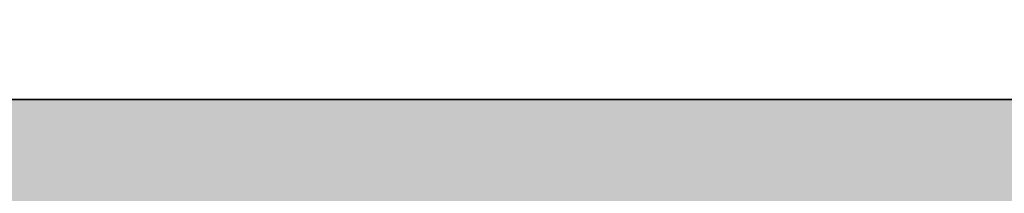
# Model space of a CAD drawing. Units: inches. Extents: x 2091 to 2899, y 967 to 2217.
# Tile 85 of 256: x 2251.283145 to 2251.287593, y 1099.918635 to 1099.919418. Entities that reach past the tile are written whole.
import ezdxf

# ---------------------------------------------------------------- set-up
doc = ezdxf.new("R2010")
doc.units = ezdxf.units.IN
doc.layers.add('A-WALL-PATT', color=141, linetype='Continuous', lineweight=13, true_color=0xadddf7)
doc.layers.add('L-SITE-WALL', color=7, linetype='Continuous', lineweight=35)

msp = doc.modelspace()

# ---------------------------------------------------------------- hatches: boundary and pattern name
at = {"layer": 'A-WALL-PATT'}
h = msp.add_hatch(color=256, dxfattribs=at)
h.dxf.hatch_style = 1
h.paths.add_polyline_path([(2212.1436027, 1941.4190588), (2387.6436027, 1941.4190588), (2387.6436027, 1824.4190588), (2392.1436027, 1824.4190588), (2392.1436027, 1941.4190588), (2609.6436027, 1941.4190588), (2609.6436027, 1825.9190588), (2614.1436027, 1825.9190588), (2614.1436027, 1941.4190588), (2794.1436027, 1941.4190588), (2794.1436027, 1928.7621663), (2803.1436027, 1928.7621663), (2803.1436027, 2050.9190588), (2203.1436027, 2050.9190588), (2203.1436027, 1900.7578592), (2212.1436027, 1900.7578592)])
h.paths.add_polyline_path([(2212.1436027, 1945.9190588), (2212.1436027, 2041.9190588), (2794.1436027, 2041.9190588), (2794.1436027, 1945.9190588), (2402.2482445, 1945.9190588), (2401.1024337, 1945.7758325), (2398.7024337, 1945.7758325)], flags=16)
h.paths.add_polyline_path([(2230.2298609, 1948.0627926), (2227.3498609, 1949.5027926), (2225.9098609, 1951.9027926), (2223.9898609, 1952.8627926), (2223.0298609, 1955.2627926), (2222.0698609, 1959.5827926), (2222.0698609, 1963.4227926), (2223.0298609, 1965.6627926), (2223.9898609, 1965.3427926), (2225.58591, 1963.860747), (2226.9115333, 1964.9572589), (2226.9488609, 1965.9387926), (2227.7783187, 1966.9521426), (2228.1999161, 1968.8787044), (2230.7098609, 1964.8627926), (2233.5898609, 1966.3027926), (2233.607309, 1966.3318728), (2233.7726595, 1964.9382048), (2234.6338015, 1963.6764729), (2235.0298609, 1963.9027926), (2236.2820348, 1965.5723578), (2235.9898609, 1962.9427926), (2237.9545121, 1957.5400019), (2238.3898609, 1957.9027926), (2239.2158609, 1960.3057926), (2238.6545655, 1966.3849599), (2238.6927918, 1966.4380694), (2238.8405779, 1967.4997069), (2238.7802908, 1967.6874864), (2238.8805378, 1967.7867629), (2238.6668609, 1966.2517926), (2239.2158609, 1960.3057926), (2238.3898609, 1957.9027926), (2236.9498609, 1956.7027926), (2234.5498609, 1949.9827926)], flags=0)
h.paths.add_polyline_path([(2278.0119735, 1948.0627926), (2276.4964266, 1947.8733492), (2275.8498328, 1947.6886081), (2274.6519735, 1947.1027926)], flags=0)
h.paths.add_polyline_path([(2269.8519735, 1955.7427926), (2268.2761762, 1956.6293287), (2270.8673022, 1956.3483982), (2269.3719735, 1958.1427926), (2268.7149641, 1959.1923253), (2270.5698328, 1958.7286081), (2268.5807252, 1961.9060872), (2270.8119735, 1960.8918835), (2270.8119735, 1963.4227926), (2271.3933148, 1964.7792556), (2270.2917623, 1966.1561963), (2271.7719735, 1965.6627926), (2272.1413868, 1966.5247568), (2273.9298328, 1965.9286081), (2275.6303855, 1968.054299), (2276.331938, 1966.72186), (2276.5204313, 1966.9521426), (2276.9420286, 1968.8787044), (2277.7342926, 1967.6110821), (2278.1398879, 1969.4645199), (2279.6591239, 1967.0337425), (2280.4119735, 1966.7827926), (2280.9493019, 1967.5887851), (2281.6098328, 1967.3686081), (2282.1332658, 1968.1537576), (2282.3492351, 1966.3334449), (2282.3498491, 1966.3325853), (2283.40755, 1968.0954201), (2283.7126314, 1965.5240203), (2284.3202211, 1964.6337894), (2284.5118085, 1964.8892393), (2284.2349735, 1965.7047926), (2284.500472, 1967.3189584), (2284.9079444, 1965.4174205), (2285.3963134, 1966.0685791), (2285.4328328, 1966.2906081), (2285.4733384, 1966.1712791), (2286.3539194, 1967.345387), (2286.2220067, 1966.1581734), (2287.6634921, 1968.0801538), (2287.7139735, 1968.4427926), (2288.4815994, 1969.0166793), (2288.5739928, 1968.7288966), (2288.9174612, 1969.0690403), (2288.6068328, 1966.8376081), (2288.9287261, 1963.3513103), (2288.9349735, 1963.3567926), (2288.9297314, 1963.3404224), (2289.015281, 1962.4138692), (2290.1112234, 1963.8751258), (2290.1328328, 1963.9426081), (2290.2176723, 1964.0170576), (2290.1112234, 1963.8751258), (2289.1558328, 1960.8916081), (2288.5940356, 1959.2572271), (2288.5719735, 1959.1027926), (2289.5319735, 1960.5427926), (2290.0119735, 1962.4627926), (2290.1918401, 1962.6426592), (2289.7698328, 1959.6886081), (2286.8898328, 1957.2886081), (2284.4898328, 1950.5686081), (2283.3146576, 1950.046308), (2283.2919735, 1949.9827926), (2280.2900585, 1948.6486081), (2281.1298328, 1948.6486081), (2282.5698328, 1948.1686081), (2283.2047262, 1948.0627926), (2278.9719735, 1948.0627926), (2276.0919735, 1949.5027926), (2274.6519735, 1951.9027926), (2272.7319735, 1952.8627926)], flags=0)
h.paths.add_polyline_path([(2271.1588684, 1958.0217654), (2272.9698328, 1955.8486081), (2272.0098328, 1960.1686081), (2272.0098328, 1964.0086081), (2272.6244258, 1965.4426583), (2274.3280226, 1963.860747), (2275.6536458, 1964.9572589), (2275.6377429, 1964.5390903), (2277.4122311, 1966.0068885), (2277.0329735, 1965.1567926), (2276.829924, 1964.9755966), (2276.7660116, 1963.2950136), (2277.4496351, 1962.6602203), (2279.4519735, 1964.8627926), (2282.3319735, 1966.3027926), (2283.5298328, 1966.8886081), (2283.2945117, 1966.7709476), (2283.9129934, 1963.8846999), (2284.8992493, 1964.4482747), (2284.7319735, 1962.9427926), (2286.6966247, 1957.5400019), (2287.1319735, 1957.9027926), (2287.5419128, 1959.0953883), (2287.7793955, 1958.4423109), (2285.6827383, 1956.6950966), (2285.8765033, 1959.7953357), (2284.7319735, 1962.9427926), (2284.8992493, 1964.4482747), (2283.9129934, 1963.8846999), (2284.2238328, 1962.4341157), (2283.4243649, 1963.6054836), (2281.6098328, 1962.5686081), (2281.1298328, 1960.1686081), (2282.0898328, 1956.3286081), (2283.0498328, 1952.9686081), (2282.5698328, 1950.5686081), (2280.1698328, 1948.6486081), (2279.883316, 1948.7918666), (2278.9719735, 1948.0627926), (2278.9719735, 1949.0227926), (2278.6723132, 1949.3973679), (2277.2898328, 1950.0886081), (2275.8498328, 1952.4886081), (2273.9298328, 1953.4486081), (2272.4898328, 1954.8886081), (2271.9216473, 1954.8886081), (2271.7719735, 1955.2627926)], flags=0)
h.paths.add_polyline_path([(2311.994146, 1955.7427926), (2312.0627174, 1955.6742211), (2312.0550999, 1955.7085002)], flags=0)
h.paths.add_polyline_path([(2331.956146, 1963.9517926), (2333.396146, 1965.3917926), (2331.077146, 1963.3567926), (2330.998603, 1963.1115166)], flags=0)
h.paths.add_polyline_path([(2310.554146, 1954.3027926), (2307.0398066, 1956.2799434), (2310.7629029, 1955.8762843), (2312.474146, 1953.8227926), (2313.434146, 1951.4227926), (2315.354146, 1950.4627926), (2316.794146, 1948.0627926), (2317.466146, 1947.7267926), (2319.3686915, 1947.9646108), (2317.754146, 1949.9827926), (2317.5695306, 1950.6104849), (2316.794146, 1951.9027926), (2314.874146, 1952.8627926), (2313.914146, 1955.2627926), (2311.514146, 1958.1427926), (2309.3754889, 1961.5591681), (2311.514146, 1960.3370783), (2311.514146, 1961.9827926), (2310.6046723, 1963.1196347), (2311.726605, 1962.4785303), (2312.4183321, 1964.09256), (2312.2559642, 1964.2955198), (2313.194146, 1963.9827926), (2313.914146, 1965.6627926), (2314.6467776, 1965.418582), (2315.354146, 1966.3027926), (2316.794146, 1967.7427926), (2316.1574354, 1966.9469043), (2317.0341105, 1965.28186), (2317.2226038, 1965.5121426), (2317.7770481, 1968.0457711), (2318.4741105, 1966.72186), (2318.6626038, 1966.9521426), (2319.0842012, 1968.8787044), (2321.2070492, 1965.4821474), (2322.1614187, 1966.9137017), (2322.554146, 1966.7827926), (2322.7859877, 1967.1305552), (2322.881646, 1966.3242926), (2323.3120408, 1965.7217399), (2323.6512889, 1965.891364), (2324.3964998, 1967.1333822), (2324.6569446, 1964.9382048), (2324.971986, 1964.476611), (2325.3872804, 1967.001499), (2325.9408127, 1964.4183481), (2327.2289286, 1966.1358361), (2327.1663199, 1965.5723578), (2328.0591386, 1966.7627827), (2328.2245759, 1966.2474864), (2329.6679714, 1967.6769101), (2329.6645759, 1967.6874864), (2329.7648229, 1967.7867629), (2329.551146, 1966.2517926), (2330.100146, 1960.3057926), (2329.3328143, 1958.0734703), (2329.3130649, 1957.935225), (2329.634146, 1958.2027926), (2330.234146, 1959.1027926), (2330.714146, 1961.0227926), (2331.034146, 1961.3427926), (2330.714146, 1959.1027926), (2329.634146, 1958.2027926), (2329.274146, 1957.6627926), (2327.7121121, 1956.3610977), (2325.434146, 1949.9827926), (2324.3337687, 1949.493736), (2323.994146, 1948.5427926), (2319.674146, 1946.6227926), (2316.794146, 1948.0627926), (2315.354146, 1950.4627926), (2313.434146, 1951.4227926)], flags=0)
h.paths.add_polyline_path([(2321.3356845, 1947.9520233), (2321.114146, 1948.0627926), (2321.114146, 1949.0227926), (2319.194146, 1951.4227926), (2316.794146, 1959.5827926), (2316.6632369, 1959.5827926), (2315.354146, 1958.1427926), (2314.394146, 1958.1427926), (2313.1483033, 1958.7090847), (2312.954146, 1959.5827926), (2312.954146, 1960.8918835), (2315.834146, 1959.5827926), (2316.6632369, 1959.5827926), (2317.3147094, 1960.2994123), (2315.0301951, 1962.420747), (2316.3558184, 1963.5172589), (2316.3723369, 1963.9516153), (2316.4701951, 1963.860747), (2317.7958184, 1964.9572589), (2317.7552187, 1963.8896871), (2319.175146, 1965.1567926), (2319.4984065, 1965.8813724), (2321.114146, 1965.3427926), (2323.2358851, 1962.3723578), (2325.6863494, 1963.7726231), (2325.5427886, 1962.4805756), (2325.1987827, 1963.4940135), (2324.4785097, 1963.0824289), (2324.9260053, 1960.9941157), (2324.0780866, 1962.2364729), (2322.4147912, 1961.2860184), (2322.074146, 1959.5827926), (2323.034146, 1955.7427926), (2323.994146, 1952.3827926), (2323.514146, 1949.9827926), (2322.1427174, 1948.8856497), (2322.074146, 1948.5427926)], flags=0)
h.paths.add_polyline_path([(2320.2074794, 1963.3374592), (2320.154146, 1963.4227926), (2320.394146, 1963.5427926)], flags=0)
h.paths.add_polyline_path([(2353.8505274, 1965.8105004), (2354.0305274, 1965.7505004), (2354.3305274, 1966.4505004), (2354.3305274, 1966.9305004)], flags=0)
h.paths.add_polyline_path([(2359.0205825, 1969.0264122), (2359.0983824, 1968.9019323), (2359.2335274, 1969.5195004), (2359.2335274, 1969.9995004)], flags=0)
h.paths.add_polyline_path([(2358.2566937, 1966.6816724), (2357.983601, 1966.3480346), (2358.211267, 1966.1461745), (2358.4104918, 1966.3895678)], flags=0)
h.paths.add_polyline_path([(2357.7684731, 1966.0587777), (2357.7321997, 1965.1049667), (2357.751047, 1965.1205565), (2357.7695274, 1965.6065004), (2357.7695274, 1966.057843)], flags=0)
h.paths.add_polyline_path([(2359.1115274, 1965.3045004), (2359.1115274, 1964.8245004), (2359.8445274, 1966.4675004), (2359.8445274, 1966.9475004)], flags=0)
h.paths.add_polyline_path([(2360.2236843, 1966.6214493), (2360.6985274, 1969.3625004), (2360.6985274, 1969.8425004), (2360.2105274, 1967.0255004), (2360.2105274, 1966.6425004)], flags=0)
h.paths.add_polyline_path([(2363.4505274, 1967.8905004), (2363.4505274, 1968.3705004), (2362.4905274, 1966.9305004), (2362.6560446, 1966.6987763)], flags=0)
h.paths.add_polyline_path([(2364.4755226, 1966.0788259), (2365.8505274, 1968.3705004), (2365.8505274, 1968.8505004), (2364.4279755, 1966.4795806)], flags=0)
h.paths.add_polyline_path([(2366.3135274, 1965.8525004), (2366.3667086, 1965.6958291), (2366.8025274, 1968.3455004), (2366.8025274, 1968.8255004)], flags=0)
h.paths.add_polyline_path([(2367.16531, 1965.8035439), (2367.2905274, 1966.9305004), (2367.2905274, 1967.4105004), (2367.1027013, 1965.7200656)], flags=0)
h.paths.add_polyline_path([(2370.0365274, 1959.9735004), (2371.0135274, 1963.0245004), (2371.0135274, 1963.5045004), (2370.0365274, 1960.4535004)], flags=0)
h.paths.add_polyline_path([(2371.6105274, 1960.2105004), (2372.5705274, 1961.6505004), (2372.5705274, 1962.1305004), (2371.8025274, 1960.9785004)], flags=0)
h.paths.add_polyline_path([(2350.8736661, 1956.0050856), (2351.9305274, 1955.8905004), (2354.4905274, 1953.3305004), (2353.8505274, 1954.9305004), (2351.4505274, 1957.8105004), (2347.9355274, 1963.4255004), (2347.9355274, 1963.9055004), (2351.4505274, 1958.2905004), (2353.7050728, 1955.5850458), (2352.8905274, 1959.2505004), (2352.8905274, 1959.7305004), (2352.8905274, 1961.9247861), (2356.7305274, 1959.7305004), (2358.454471, 1961.6268384), (2354.8105274, 1965.0105004), (2355.0308552, 1965.2859102), (2358.6910907, 1961.8871201), (2361.5305274, 1965.0105004), (2364.3764954, 1966.4334844), (2364.5243939, 1965.1869106), (2365.454468, 1963.8241807), (2365.8810728, 1964.0679549), (2365.3705274, 1966.4505004), (2365.3705274, 1966.9305004), (2366.8105274, 1960.2105004), (2366.8105274, 1959.7305004), (2366.3887092, 1952.9814095), (2367.7705274, 1956.8505004), (2368.641225, 1957.5760818), (2366.8105274, 1962.6105004), (2366.8105274, 1963.0905004), (2368.7751785, 1957.6877097), (2369.2105274, 1958.0505004), (2370.0015924, 1960.3518674), (2369.4752319, 1966.0526677), (2369.5134582, 1966.1057772), (2369.514173, 1966.1109121), (2369.4752319, 1966.5326677), (2369.5134582, 1966.5857772), (2369.614635, 1967.3125914), (2369.1825274, 1968.6585004), (2369.1825274, 1969.1385004), (2369.6009573, 1967.8351942), (2369.7012042, 1967.9344708), (2369.7179468, 1968.054743), (2370.1451758, 1968.3741448), (2369.7787075, 1968.0112238), (2369.7012042, 1967.4544708), (2370.4681613, 1968.2140038), (2369.674936, 1967.2657706), (2369.514173, 1966.1109121), (2370.0365274, 1960.4535004), (2370.0365274, 1959.9735004), (2369.441756, 1958.2431909), (2370.6505274, 1959.2505004), (2371.0458215, 1962.0175592), (2371.1305274, 1962.1305004), (2370.6505274, 1958.7705004), (2367.7705274, 1956.3705004), (2365.3705274, 1949.6505004), (2362.0790988, 1948.1876432), (2363.4505274, 1947.7305004), (2361.0505274, 1947.7305004), (2360.0905274, 1947.7305004), (2357.1038607, 1947.3571671), (2360.0905274, 1948.2105004), (2358.1705274, 1949.1705004), (2356.7305274, 1951.5705004), (2354.8105274, 1952.5305004), (2351.9305274, 1955.4105004)], flags=0)
h.paths.add_polyline_path([(2361.0505274, 1948.6905004), (2359.1305274, 1951.0905004), (2356.7305274, 1959.2505004), (2355.7705274, 1959.2505004), (2352.8905274, 1960.5595913), (2352.8905274, 1961.4447861), (2355.8905274, 1959.7305004), (2356.7305274, 1959.7305004), (2356.837194, 1959.3678337), (2361.5305274, 1964.5305004), (2363.2484221, 1965.3894478), (2364.92531, 1963.0418047), (2362.4905274, 1961.6505004), (2362.0638607, 1959.5171671), (2362.9705274, 1955.8905004), (2363.9305274, 1952.5305004), (2363.9305274, 1952.0505004), (2363.4505274, 1949.6505004), (2361.0505274, 1947.7305004)], flags=0)
h.paths.add_polyline_path([(2359.1305274, 1951.5705004), (2359.2905274, 1951.3705004), (2361.0505274, 1954.4505004), (2361.0505274, 1954.9305004)], flags=0)
h.paths.add_polyline_path([(2357.2195274, 1966.5455004), (2356.7925274, 1968.8145004), (2356.7925274, 1969.2945004), (2357.2195274, 1967.0255004)], flags=0)
h.paths.add_polyline_path([(2361.0505274, 1954.4505004), (2361.5305274, 1958.7705004), (2361.5305274, 1959.2505004), (2361.0505274, 1954.9305004)], flags=0)
h.paths.add_polyline_path([(2402.5482874, 1948.4860764), (2402.3024337, 1948.4158325), (2402.5904337, 1948.4158325)], flags=0)
h.paths.add_polyline_path([(2394.1424337, 1956.0958325), (2395.6850518, 1954.5532144), (2396.7204952, 1953.9706788), (2396.0624337, 1955.6158325), (2395.2413811, 1956.6010956), (2395.8789043, 1956.4417148), (2395.1024337, 1959.9358325), (2395.1024337, 1963.7758325), (2396.0624337, 1966.0158325), (2397.0224337, 1965.6958325), (2398.6184828, 1964.2137869), (2399.9441061, 1965.3102988), (2399.9814337, 1966.2918325), (2400.8108915, 1967.3051825), (2401.2324888, 1969.2317443), (2403.5379492, 1965.5430077), (2403.9419843, 1967.3893156), (2404.7024337, 1967.1358325), (2405.4603284, 1966.0747799), (2406.6224337, 1966.6558325), (2406.6398818, 1966.6849127), (2406.8052323, 1965.2912447), (2406.9256943, 1965.1147456), (2407.3424337, 1964.9758325), (2407.8743256, 1965.7736703), (2408.1691004, 1964.3980547), (2409.3146076, 1965.9253977), (2409.2174583, 1965.0510538), (2409.4452323, 1963.1312447), (2410.3063743, 1961.8695128), (2410.7024337, 1962.0958325), (2411.4422687, 1963.0822792), (2411.1654337, 1963.8978325), (2411.6164263, 1966.6397566), (2411.7253645, 1966.7911093), (2411.8731507, 1967.8527468), (2411.8128636, 1968.0405263), (2411.9131106, 1968.1398028), (2411.6994337, 1966.6048325), (2412.2484337, 1960.6588325), (2413.2254337, 1963.7098325), (2414.3779002, 1964.7211603), (2414.5131507, 1965.6927468), (2414.4528636, 1965.8805263), (2414.5531106, 1965.9798028), (2414.3779002, 1964.7211603), (2414.5198172, 1964.8456973), (2414.3653645, 1964.6311093), (2414.3394337, 1964.4448325), (2414.8884337, 1958.4988325), (2414.0624337, 1956.0958325), (2412.6224337, 1954.8958325), (2410.1713699, 1948.0328538), (2410.0167194, 1948.0844039), (2405.9024337, 1946.2558325), (2405.9024337, 1947.2158325), (2405.2042519, 1948.0885598), (2404.2224337, 1948.4158325), (2403.2624337, 1948.4158325), (2400.3824337, 1949.8558325), (2399.6624337, 1951.0558325), (2397.9824337, 1952.7358325), (2397.0224337, 1953.2158325), (2395.6850518, 1954.5532144), (2392.6567764, 1956.2569078)], flags=0)
h.paths.add_polyline_path([(2409.0856501, 1964.4074407), (2409.1303635, 1964.2757154), (2409.2624337, 1964.4958325)], flags=0)
h.paths.add_polyline_path([(2397.7424337, 1961.6158325), (2398.7024337, 1963.8558325), (2399.6624337, 1963.5358325), (2401.4265631, 1965.7409942), (2401.7914151, 1966.5588003), (2402.0714337, 1965.0708325), (2402.8355074, 1964.3933667), (2403.2623982, 1964.9148999), (2403.3381187, 1964.771086), (2402.6155159, 1963.9762229), (2402.4986125, 1960.9022379), (2403.5429971, 1959.9324522), (2404.4132029, 1960.8896786), (2404.7024337, 1962.3358325), (2407.9163468, 1964.1723542), (2409.5202115, 1961.9269436), (2410.9870849, 1957.8930418), (2411.4224337, 1958.2558325), (2412.0479637, 1960.075625), (2412.4103407, 1959.0790883), (2411.6756205, 1958.4668215), (2411.6624337, 1958.2558325), (2411.6260701, 1958.4255295), (2409.9824337, 1957.0558325), (2407.5824337, 1950.3358325), (2403.2624337, 1948.4158325), (2403.2624337, 1949.3758325), (2401.3424337, 1951.7758325), (2399.4165078, 1958.3239806), (2397.7424337, 1959.0849234), (2397.7424337, 1959.9701182), (2397.1024337, 1960.3358325), (2397.7424337, 1960.0449234)], flags=0)
h.paths.add_polyline_path([(2405.9024337, 1952.9758325), (2405.9504337, 1953.4078325), (2406.0167194, 1953.1758325)], flags=0)
h.paths.add_polyline_path([(2449.817778, 1967.1140143), (2449.7523235, 1967.1358325), (2449.7937028, 1967.0779014)], flags=0)
h.paths.add_polyline_path([(2451.6976961, 1966.6181202), (2451.7408949, 1966.6901182), (2451.6920515, 1966.6656965)], flags=0)
h.paths.add_polyline_path([(2454.3436278, 1965.7375716), (2455.7523235, 1967.6158325), (2455.9923235, 1968.0958325), (2454.3644974, 1965.9253977)], flags=0)
h.paths.add_polyline_path([(2457.5473235, 1968.8638325), (2457.7873235, 1969.3438325), (2457.0543235, 1968.7958325), (2457.0076216, 1968.4603446)], flags=0)
h.paths.add_polyline_path([(2456.9217835, 1967.8566619), (2456.8022381, 1968.2290163), (2456.7230003, 1967.6598028)], flags=0)
h.paths.add_polyline_path([(2457.3023235, 1967.3768325), (2457.5423235, 1967.8568325), (2456.8103235, 1966.8398325), (2456.7405164, 1966.7002183), (2456.7490213, 1966.6081053)], flags=0)
h.paths.add_polyline_path([(2458.2753235, 1963.7098325), (2458.1553426, 1963.3351533), (2460.3543235, 1965.2648325), (2460.5943235, 1965.7448325)], flags=0)
h.paths.add_polyline_path([(2458.3923235, 1962.8158325), (2458.3640882, 1962.6181854), (2459.5923235, 1964.2558325), (2459.8323235, 1964.7358325)], flags=0)
h.paths.add_polyline_path([(2459.3523235, 1962.8158325), (2459.2723235, 1962.4958325), (2460.0723235, 1963.2958325), (2460.3123235, 1963.7758325)], flags=0)
h.paths.add_polyline_path([(2458.6803235, 1960.6078325), (2458.6323235, 1960.4158325), (2459.5923235, 1961.8558325), (2459.8323235, 1962.3358325)], flags=0)
h.paths.add_polyline_path([(2437.8381696, 1956.2426502), (2439.1923235, 1956.0958325), (2441.3523235, 1953.9358325), (2440.8723235, 1955.1358325), (2438.4723235, 1958.0158325), (2438.0715634, 1958.6560225), (2438.7123235, 1958.4958325), (2440.6395962, 1956.1831052), (2439.9123235, 1959.4558325), (2439.9123235, 1963.2958325), (2441.3523235, 1966.6558325), (2441.5923235, 1967.1358325), (2441.1123235, 1966.0158325), (2442.0723235, 1965.6958325), (2443.9889932, 1968.0916696), (2444.2413235, 1966.7508325), (2444.9168011, 1966.1519203), (2445.6765737, 1967.0801359), (2446.2553235, 1969.7248325), (2446.4953235, 1970.2048325), (2446.2823786, 1969.2317443), (2447.362672, 1967.5032748), (2447.7203235, 1969.5678325), (2447.9603235, 1970.0478325), (2447.4854804, 1967.3067814), (2448.7923235, 1965.2158325), (2448.4723235, 1964.8638325), (2448.5523235, 1964.7358325), (2451.4520515, 1966.1856965), (2451.615122, 1964.8112447), (2452.3079173, 1963.7961718), (2453.2345053, 1964.3256507), (2454.0723235, 1960.4158325), (2453.6286871, 1953.3176507), (2454.7923235, 1956.5758325), (2455.0323235, 1957.0558325), (2455.7188351, 1957.6279255), (2453.8323235, 1962.8158325), (2453.940966, 1963.7936155), (2453.3353235, 1965.5778325), (2453.8243235, 1968.5508325), (2454.0643235, 1969.0308325), (2453.5753235, 1966.0578325), (2454.0403331, 1964.6879188), (2453.8323235, 1962.8158325), (2455.7188351, 1957.6279255), (2456.3672068, 1958.1682353), (2457.0583235, 1960.1788325), (2457.2983235, 1960.6588325), (2456.4723235, 1958.2558325), (2457.7177289, 1959.2936703), (2457.6723235, 1958.9758325), (2454.8899506, 1956.6571884), (2453.6141416, 1953.0849234), (2453.5923235, 1952.7358325), (2453.3523235, 1952.2558325), (2453.3595962, 1952.3721961), (2452.6323235, 1950.3358325), (2452.3923235, 1949.8558325), (2449.203752, 1948.4386896), (2450.7123235, 1947.9358325), (2448.0723235, 1947.9358325), (2447.1123235, 1947.9358325), (2444.5523235, 1947.6158325), (2447.1995962, 1948.3721961), (2445.1923235, 1949.3758325), (2443.7523235, 1951.7758325), (2441.8323235, 1952.7358325), (2438.9523235, 1955.6158325)], flags=0)
h.paths.add_polyline_path([(2443.9923235, 1959.9358325), (2444.0403235, 1959.7726325), (2444.1215542, 1959.8619863)], flags=0)
h.paths.add_polyline_path([(2442.9123235, 1959.9358325), (2443.0323235, 1959.9358325), (2442.4456568, 1960.2024992)], flags=0)
h.paths.add_polyline_path([(2444.9829435, 1965.0196767), (2445.2793235, 1965.2648325), (2445.5193235, 1965.7448325), (2444.9939958, 1965.3102988)], flags=0)
h.paths.add_polyline_path([(2446.1333235, 1965.0298325), (2446.3303662, 1965.4714986), (2444.9703235, 1964.2578325), (2444.7303235, 1963.7778325)], flags=0)
h.paths.add_polyline_path([(2442.7923235, 1959.4558325), (2443.7523235, 1959.4558325), (2446.1523235, 1951.2958325), (2446.4123235, 1951.7508325), (2446.3923235, 1951.7758325), (2448.0805993, 1954.7303152), (2448.5523235, 1958.9758325), (2441.8323235, 1965.2158325), (2442.1549464, 1965.6191112), (2448.7923235, 1959.4558325), (2448.3123235, 1955.1358325), (2448.0723235, 1954.6558325), (2446.4123235, 1951.7508325), (2448.3123235, 1949.3758325), (2448.3123235, 1948.4158325), (2450.5408949, 1950.1986896), (2450.9523235, 1952.2558325), (2449.9923235, 1955.6158325), (2449.0323235, 1959.4558325), (2449.5123235, 1961.8558325), (2449.7523235, 1962.3358325), (2449.6749041, 1961.9487357), (2452.9945053, 1963.8456507), (2453.0644143, 1963.5194086), (2452.8846108, 1963.7828538), (2449.6749041, 1961.9487357), (2449.2723235, 1959.9358325), (2450.2323235, 1956.0958325), (2451.1923235, 1952.7358325), (2450.7123235, 1950.3358325), (2450.4723235, 1949.8558325), (2448.0723235, 1947.9358325), (2448.0723235, 1948.5358325), (2445.4323235, 1949.8558325), (2443.9923235, 1952.2558325), (2442.0723235, 1953.2158325), (2441.1123235, 1955.6158325), (2440.1523235, 1959.9358325), (2440.1523235, 1960.6558325)], flags=0)
h.paths.add_polyline_path([(2456.6923235, 1966.9858325), (2457.6083235, 1968.0808325), (2457.8483235, 1968.5608325), (2456.9323235, 1967.4658325)], flags=0)
h.paths.add_polyline_path([(2489.8965704, 1966.5802407), (2489.9429477, 1966.1893466), (2490.7474884, 1967.5302478), (2491.3191223, 1968.9511605)], flags=0)
h.paths.add_polyline_path([(2473.5624709, 1956.4071313), (2477.139981, 1956.0192567), (2476.955333, 1956.2408343), (2475.1080486, 1957.2801078), (2476.3474884, 1956.9702478), (2475.1869011, 1958.8242158), (2476.9191223, 1958.3911605), (2475.4116422, 1960.7992688), (2477.7874884, 1959.7193388), (2477.7874884, 1962.2502478), (2477.637399, 1962.4378595), (2477.8225502, 1962.3320588), (2478.3591223, 1963.5840603), (2478.3591223, 1963.6711605), (2477.3243485, 1964.9646278), (2478.7148258, 1964.5011354), (2479.3191223, 1965.9111605), (2480.2791223, 1965.5911605), (2481.7839654, 1967.4722144), (2482.1164884, 1965.7052478), (2482.8805621, 1965.027782), (2483.209305, 1965.4294079), (2483.2201695, 1965.7150902), (2483.0759397, 1965.9890218), (2483.7117624, 1966.7658076), (2484.1304884, 1968.6792478), (2484.7021223, 1970.1001605), (2484.4891774, 1969.1270723), (2486.5029044, 1965.9051092), (2487.3874884, 1965.6102478), (2488.1534195, 1966.7591445), (2488.717017, 1965.9701079), (2489.2000857, 1966.2116422), (2489.3306713, 1965.1109919), (2490.3939049, 1963.6224649), (2490.6607651, 1963.7749564), (2490.4939052, 1964.553636), (2490.9230629, 1963.9248409), (2491.3191223, 1964.1511605), (2491.3333892, 1964.1701831), (2491.2104884, 1964.5322478), (2491.2817559, 1964.9655369), (2491.425789, 1964.2933827), (2494.0764757, 1967.8276317), (2494.4979183, 1966.5149416), (2494.5981652, 1966.6142182), (2494.6894884, 1967.2702478), (2495.106748, 1967.5821964), (2495.1298393, 1967.7480749), (2495.0695522, 1967.9358543), (2495.1697991, 1968.0351309), (2495.0317768, 1967.0436325), (2495.7538179, 1967.7586844), (2494.9820531, 1966.6864374), (2494.9561223, 1966.5001605), (2495.4790212, 1960.8368513), (2495.9104884, 1962.1842478), (2496.4821223, 1963.6051605), (2496.0726945, 1962.3265891), (2496.7689042, 1962.9375364), (2496.5991223, 1962.7111605), (2496.1191223, 1959.3511605), (2496.7328731, 1960.2717868), (2496.9874884, 1961.2902478), (2497.5591223, 1962.7111605), (2497.0791223, 1960.7911605), (2496.5074884, 1959.3702478), (2495.5474884, 1957.9302478), (2492.7588421, 1955.6063759), (2490.8391223, 1950.2311605), (2490.2674884, 1948.8102478), (2485.9474884, 1946.8902478), (2483.0674884, 1948.3302478), (2481.6274884, 1950.7302478), (2479.7074884, 1951.6902478), (2476.8274884, 1954.5702478)], flags=0)
h.paths.add_polyline_path([(2485.5769732, 1948.3133919), (2485.5591223, 1948.3111605), (2485.5787582, 1948.3111605)], flags=0)
h.paths.add_polyline_path([(2478.6450633, 1954.5511605), (2478.1090419, 1956.963257), (2479.3191223, 1955.5111605), (2480.2791223, 1953.1111605), (2482.1991223, 1952.1511605), (2483.6391223, 1949.7511605), (2486.5191223, 1948.3111605), (2486.5191223, 1949.2711605), (2484.7393067, 1951.49593), (2484.0274884, 1950.2502478), (2481.6274884, 1958.4102478), (2482.3751479, 1959.2326733), (2482.1991223, 1959.8311605), (2483.1975724, 1960.9294556), (2479.7074884, 1964.1702478), (2480.6033578, 1965.2900847), (2481.8751714, 1964.109115), (2482.666387, 1964.7635825), (2482.6153591, 1963.4217978), (2482.9891988, 1963.0746609), (2484.0084884, 1963.9842478), (2484.6836065, 1965.4975071), (2484.5801223, 1965.4051605), (2485.3572683, 1967.1471126), (2485.1206453, 1965.7811968), (2486.4274884, 1963.6902478), (2488.1453831, 1964.5491952), (2489.822271, 1962.2015522), (2490.7474884, 1962.7302478), (2491.9996623, 1964.3998131), (2492.0760458, 1965.0872647), (2492.2128915, 1964.6841187), (2492.4853744, 1965.0474291), (2492.2791223, 1963.1911605), (2494.2437735, 1957.7883698), (2494.5625035, 1958.0539782), (2494.9334884, 1959.1332478), (2495.5051223, 1960.5541605), (2494.6791223, 1958.1511605), (2494.1074884, 1956.7302478), (2494.5625035, 1958.0539782), (2493.4085439, 1957.0923452), (2491.7074884, 1961.7702478), (2491.9996623, 1964.3998131), (2490.7474884, 1962.7302478), (2487.7120303, 1960.9957003), (2487.4791223, 1959.8311605), (2488.4391223, 1955.9911605), (2489.3991223, 1952.6311605), (2488.9191223, 1950.2311605), (2488.5769183, 1949.9573973), (2488.3474884, 1948.8102478), (2487.6517154, 1948.2536295), (2487.4791223, 1948.3111605), (2486.5191223, 1948.3111605), (2483.6391223, 1949.7511605), (2482.1991223, 1952.1511605), (2480.2791223, 1953.1111605), (2478.8391223, 1954.5511605)], flags=0)
h.paths.add_polyline_path([(2526.648252, 1966.9875242), (2526.5173429, 1967.0311605), (2526.6001016, 1966.9152985)], flags=0)
h.paths.add_polyline_path([(2528.4706401, 1966.4466558), (2528.5744858, 1966.619732), (2528.4570709, 1966.5610245)], flags=0)
h.paths.add_polyline_path([(2534.1333429, 1967.4961605), (2534.1566852, 1967.5428451), (2534.0598415, 1967.4082958)], flags=0)
h.paths.add_polyline_path([(2536.1619229, 1964.0506005), (2535.1573429, 1962.7111605), (2535.1008723, 1962.3158664), (2536.1173429, 1963.6711605), (2536.4205319, 1964.2775386)], flags=0)
h.paths.add_polyline_path([(2535.1573429, 1959.8311605), (2536.1173429, 1961.2711605), (2536.5973429, 1962.2311605), (2535.2533429, 1960.2151605)], flags=0)
h.paths.add_polyline_path([(2513.2490352, 1956.284796), (2516.2211807, 1955.9625552), (2514.9973429, 1957.4311605), (2514.1958227, 1958.7115406), (2515.4773429, 1958.3911605), (2516.9318884, 1956.645706), (2516.4373429, 1958.8711605), (2516.4373429, 1962.7111605), (2516.8726918, 1963.7269745), (2515.3464338, 1965.6347969), (2517.3973429, 1964.9511605), (2517.8773429, 1966.0711605), (2518.3573429, 1967.0311605), (2517.8773429, 1965.9111605), (2518.8373429, 1965.5911605), (2520.4865896, 1967.6527188), (2520.7663429, 1966.1661605), (2521.5304166, 1965.4886947), (2521.7814433, 1965.7953745), (2521.8009106, 1966.307268), (2521.4778037, 1966.9209358), (2521.2463429, 1967.1261605), (2521.1777006, 1967.4909132), (2521.4778037, 1966.9209358), (2522.0104166, 1966.4486947), (2522.2573857, 1966.7504173), (2522.7803429, 1969.1401605), (2523.2603429, 1970.1001605), (2523.0473981, 1969.1270723), (2524.6731324, 1966.5258974), (2526.0373429, 1966.0711605), (2526.7952377, 1965.0101079), (2527.9770709, 1965.6010245), (2528.1401415, 1964.2265727), (2528.6645901, 1963.4581589), (2529.3886157, 1963.8718878), (2529.3296653, 1964.1469896), (2529.4812835, 1963.9248409), (2529.8773429, 1964.1511605), (2529.9840096, 1964.2933827), (2529.7890531, 1965.2031796), (2530.0623998, 1964.397903), (2532.802483, 1968.0513473), (2533.1477728, 1966.9758543), (2533.2480198, 1967.0751309), (2533.3393429, 1967.7311605), (2533.6728477, 1967.9804929), (2533.7280198, 1968.0351309), (2533.5143429, 1966.5001605), (2534.0247176, 1960.9724963), (2534.5603429, 1962.6451605), (2535.0403429, 1963.6051605), (2534.0633429, 1960.5541605), (2533.2373429, 1958.1511605), (2534.2881537, 1959.0268362), (2534.1973429, 1958.3911605), (2531.5125972, 1956.1538724), (2529.3973429, 1950.2311605), (2528.9173429, 1949.2711605), (2526.4487715, 1948.1740177), (2527.4773429, 1947.8311605), (2530.3573429, 1947.3511605), (2524.5973429, 1947.3511605), (2521.7173429, 1948.7911605), (2520.2773429, 1951.1911605), (2518.3573429, 1952.1511605), (2515.4773429, 1955.0311605)], flags=0)
h.paths.add_polyline_path([(2523.9347601, 1967.1903084), (2523.6195125, 1966.4836893), (2523.7704999, 1966.2421094)], flags=0)
h.paths.add_polyline_path([(2518.8373429, 1953.1111605), (2517.8773429, 1955.5111605), (2516.8849834, 1959.9767785), (2516.9173429, 1959.9620696), (2516.9173429, 1962.0254462), (2520.7573429, 1959.8311605), (2522.0249486, 1961.2255267), (2518.3573429, 1964.6311605), (2519.0025888, 1965.4377179), (2520.433392, 1964.109115), (2521.3011199, 1964.8268709), (2521.2451575, 1963.3553327), (2525.6383068, 1959.2759798), (2526.0373429, 1961.2711605), (2529.3973429, 1963.1911605), (2530.6495168, 1964.8607257), (2530.6647196, 1964.9975502), (2530.6919561, 1964.9173115), (2531.0877777, 1965.4450736), (2530.9459855, 1964.1689435), (2530.6919561, 1964.9173115), (2529.3973429, 1963.1911605), (2526.3625042, 1961.456967), (2526.0373429, 1959.8311605), (2526.9973429, 1955.9911605), (2527.9573429, 1952.6311605), (2527.4773429, 1950.2311605), (2527.1344858, 1949.9568748), (2526.9739283, 1949.1540874), (2526.6973429, 1949.0311605), (2524.5973429, 1947.3511605), (2524.5973429, 1948.3111605), (2524.2773429, 1948.7111605), (2522.1973429, 1949.7511605), (2520.7573429, 1952.1511605)], flags=0)
h.paths.add_polyline_path([(2520.2773429, 1958.8711605), (2520.8533429, 1959.5047605), (2523.1573429, 1951.6711605), (2524.6138947, 1954.220126), (2524.5973429, 1954.0711605), (2522.6773429, 1950.7111605)], flags=0)
h.paths.add_polyline_path([(2559.3709104, 1966.3111605), (2559.3984114, 1966.324911), (2559.4019428, 1966.3452961)], flags=0)
h.paths.add_polyline_path([(2549.7709104, 1957.1911605), (2552.6509104, 1954.3111605), (2552.1339874, 1955.6034682), (2550.6109104, 1957.4311605), (2547.0959104, 1963.0461605), (2545.7759104, 1965.2061605), (2549.2909104, 1959.5911605), (2551.6909104, 1956.7111605), (2550.7929329, 1960.7520594), (2550.7309104, 1960.7802514), (2550.7309104, 1964.8711605), (2551.6909104, 1967.1111605), (2552.6509104, 1966.7911605), (2554.2469595, 1965.309115), (2555.0342517, 1965.9603371), (2555.5816714, 1966.6446117), (2555.6099104, 1967.3871605), (2556.4393682, 1968.4005106), (2556.8609656, 1970.3270723), (2559.3709104, 1966.3111605), (2560.6909104, 1964.1511605), (2562.4088052, 1965.0101079), (2561.6509104, 1966.0711605), (2560.3309104, 1968.2311605), (2561.7584966, 1966.2325398), (2562.3472126, 1967.1156138), (2562.433709, 1966.3865727), (2563.127798, 1965.3696043), (2563.5709104, 1965.5911605), (2563.5883585, 1965.6202407), (2563.3625433, 1967.5235403), (2563.7224894, 1965.8437921), (2565.0600013, 1968.0729787), (2564.7328616, 1965.1287215), (2565.1175771, 1963.3333827), (2567.4446216, 1966.4361087), (2567.315615, 1967.8333279), (2567.3538413, 1967.8864374), (2567.5016274, 1968.9480749), (2567.4413403, 1969.1358543), (2567.5415873, 1969.2351309), (2567.3279104, 1967.7001605), (2567.8769104, 1961.7541605), (2568.7466892, 1964.4703273), (2568.635615, 1965.6733279), (2568.6738413, 1965.7264374), (2568.8216274, 1966.7880749), (2568.7613403, 1966.9758543), (2568.8615873, 1967.0751309), (2568.6479104, 1965.5401605), (2568.7261271, 1964.6930264), (2568.8539104, 1964.8051605), (2568.7466892, 1964.4703273), (2568.8172361, 1963.7062615), (2568.9709104, 1963.9111605), (2568.8660747, 1963.1773104), (2569.1969104, 1959.5941605), (2568.3709104, 1957.1911605), (2566.9309104, 1955.9911605), (2564.6202721, 1949.5213733), (2564.6509104, 1949.5111605), (2564.6166247, 1949.5111605), (2564.5309104, 1949.2711605), (2560.2109104, 1947.3511605), (2557.3309104, 1948.7911605), (2556.0451961, 1950.9340177), (2556.0109104, 1950.9511605), (2555.8566247, 1951.2083034), (2553.9709104, 1952.1511605), (2551.0909104, 1955.0311605), (2546.6501439, 1957.5295149)], flags=0)
h.paths.add_polyline_path([(2567.0257941, 1959.3302303), (2567.0350071, 1959.3048946), (2567.0509104, 1959.3511605)], flags=0)
h.paths.add_polyline_path([(2551.9682875, 1962.5183736), (2553.0109104, 1964.9511605), (2553.9709104, 1964.6311605), (2555.5669595, 1963.149115), (2556.8925828, 1964.2456268), (2556.9299104, 1965.2271605), (2557.1439841, 1965.4886947), (2556.420066, 1966.1305566), (2556.3914211, 1966.1049947), (2556.3799104, 1966.1661605), (2556.420066, 1966.1305566), (2556.9519104, 1966.6051605), (2557.0921386, 1966.9194783), (2557.5708749, 1966.010228), (2557.7593682, 1966.2405106), (2557.4179104, 1964.6801605), (2556.8925828, 1964.2456268), (2556.8070892, 1961.997566), (2560.6909104, 1958.3911605), (2560.6355258, 1957.892699), (2560.8109104, 1957.1911605), (2561.7709104, 1953.8311605), (2561.2909104, 1951.4311605), (2559.1104226, 1949.6867703), (2559.1564842, 1949.6291933), (2563.0265202, 1951.3492093), (2562.6109104, 1949.2711605), (2560.2109104, 1947.3511605), (2560.2109104, 1948.3111605), (2559.2509104, 1949.5111605), (2558.8909104, 1949.5111605), (2558.8909104, 1949.9611605), (2558.2909104, 1950.7111605), (2558.0537011, 1951.5176722), (2556.9709104, 1952.8711605), (2555.0678801, 1959.3414636), (2552.0509104, 1961.0654462), (2552.0509104, 1962.4711605)], flags=0)
h.paths.add_polyline_path([(2588.3300486, 1958.3911605), (2588.6102476, 1958.1109615), (2588.5533615, 1958.3669489)], flags=0)
h.paths.add_polyline_path([(2594.745454, 1950.4930862), (2593.9575317, 1953.1720221), (2593.1300486, 1954.5511605), (2591.2100486, 1955.5111605), (2590.2500486, 1957.9111605), (2588.3090328, 1960.2403795), (2586.1773061, 1961.2093462), (2587.8500486, 1960.7911605), (2587.2534157, 1961.7442456), (2588.4413145, 1961.0654462), (2588.4413145, 1962.6555276), (2588.4216793, 1962.6653452), (2588.4413145, 1962.7111605), (2586.9140379, 1964.6202563), (2588.8770864, 1963.7279616), (2589.2900486, 1964.6915402), (2589.2900486, 1966.0711605), (2590.2500486, 1968.3111605), (2591.2100486, 1967.9911605), (2592.8060977, 1966.509115), (2594.131721, 1967.6056268), (2594.1690486, 1968.5871605), (2594.9985064, 1969.6005106), (2595.4201038, 1971.5270723), (2597.9300486, 1967.5111605), (2600.8100486, 1968.9511605), (2600.8274967, 1968.9802407), (2600.9928472, 1967.5865727), (2601.8539892, 1966.3248409), (2602.1071433, 1966.4695004), (2602.2363539, 1967.255069), (2602.3567153, 1966.6933827), (2603.5022225, 1968.2207257), (2603.2100486, 1965.5911605), (2605.1746998, 1960.1883698), (2605.506891, 1960.4651958), (2605.026019, 1965.6733279), (2605.0642453, 1965.7264374), (2605.2120315, 1966.7880749), (2605.1517444, 1966.9758543), (2605.2519913, 1967.0751309), (2605.3433145, 1967.7311605), (2605.9529049, 1968.1868979), (2605.8747531, 1969.0333279), (2605.9129794, 1969.0864374), (2606.0607656, 1970.1480749), (2606.0004785, 1970.3358543), (2606.1007255, 1970.4351309), (2605.8870486, 1968.9001605), (2606.4360486, 1962.9541605), (2605.6100486, 1960.5511605), (2605.9970364, 1960.8736504), (2606.5643145, 1962.6451605), (2608.2414939, 1964.1169415), (2608.0100486, 1963.1911605), (2607.0500486, 1961.7511605), (2606.6314856, 1961.402358), (2606.2013145, 1958.3911605), (2603.3213145, 1955.9911605), (2600.9213145, 1949.2711605), (2596.6013145, 1947.3511605), (2593.7213145, 1948.7911605), (2592.8573145, 1950.2311605), (2592.6500486, 1950.2311605)], flags=0)
h.paths.add_polyline_path([(2596.6013145, 1947.3511605), (2596.6013145, 1948.3111605), (2594.6813145, 1950.7111605), (2596.1549537, 1953.2900292), (2595.5300486, 1954.0711605), (2593.1992262, 1961.9959568), (2592.6513399, 1962.5047084), (2591.780151, 1963.0025306), (2593.2829868, 1964.2456268), (2593.3203145, 1965.2271605), (2594.1497723, 1966.2405106), (2594.5713696, 1968.1670723), (2596.1826506, 1965.5890227), (2596.9512732, 1966.4345076), (2598.0413145, 1966.0711605), (2598.7992092, 1965.0101079), (2599.9613145, 1965.5911605), (2599.9787626, 1965.6202407), (2600.144113, 1964.2265727), (2601.0052551, 1962.9648409), (2601.4013145, 1963.1911605), (2602.6534884, 1964.8607257), (2602.3613145, 1962.2311605), (2603.7927479, 1958.2947186), (2601.9776436, 1953.2124265), (2601.9462078, 1952.7094535), (2599.4687551, 1951.6083634), (2599.0013145, 1949.2711605)], flags=0)
h.paths.add_polyline_path([(2597.5613145, 1958.8711605), (2597.6709663, 1959.4194194), (2597.5950535, 1958.7362045)], flags=0)
h.paths.add_polyline_path([(2623.6663046, 1961.2543751), (2625.5191629, 1960.7911605), (2624.9655444, 1961.6755326), (2627.1991629, 1960.6602514), (2627.1991629, 1961.1511605), (2626.9591629, 1962.2311605), (2626.9591629, 1963.4911605), (2625.5823208, 1965.2122132), (2626.9591629, 1964.4254462), (2626.9591629, 1965.8311605), (2626.8691629, 1965.8611605), (2627.9191629, 1968.3111605), (2628.8791629, 1967.9911605), (2630.475212, 1966.509115), (2631.8008353, 1967.6056268), (2631.8381629, 1968.5871605), (2632.6676207, 1969.6005106), (2633.089218, 1971.5270723), (2635.5991629, 1967.5111605), (2638.4791629, 1968.9511605), (2638.496611, 1968.9802407), (2638.6619615, 1967.5865727), (2639.1762733, 1966.8330111), (2639.7802155, 1967.8395816), (2640.0258296, 1966.6933827), (2641.1713368, 1968.2207257), (2640.8791629, 1965.5911605), (2641.114265, 1964.9446299), (2641.4113368, 1965.3407257), (2641.3080991, 1964.4115861), (2642.8438141, 1960.1883698), (2643.2791629, 1960.5511605), (2644.0847364, 1962.8947358), (2643.7838674, 1966.1533279), (2643.8068345, 1966.185237), (2643.6006764, 1968.418053), (2643.5228121, 1968.6605812), (2643.7298799, 1970.1480749), (2643.6695928, 1970.3358543), (2643.7698398, 1970.4351309), (2643.5561629, 1968.9001605), (2643.6006764, 1968.418053), (2643.9095928, 1967.4558543), (2644.0098398, 1967.5551309), (2643.8117426, 1966.1320789), (2644.1051629, 1962.9541605), (2644.2387733, 1961.3508359), (2644.7191629, 1961.7511605), (2645.0328526, 1962.2216951), (2645.3221629, 1963.1251605), (2646.0764203, 1963.7870466), (2645.0328526, 1962.2216951), (2644.3451629, 1960.0741605), (2643.5191629, 1957.6711605), (2642.0791629, 1956.4711605), (2639.7196124, 1949.864419), (2639.8755265, 1949.8384333), (2635.3591629, 1947.8311605), (2632.4791629, 1949.2711605), (2631.0391629, 1951.6711605), (2629.1191629, 1952.6311605), (2628.1591629, 1955.0311605), (2625.7591629, 1957.9111605)], flags=0)
h.paths.add_polyline_path([(2627.8163058, 1956.5740177), (2627.3737084, 1958.565706), (2626.3763058, 1959.7625891), (2627.1991629, 1959.3511605), (2627.3737084, 1958.565706), (2627.9191629, 1957.9111605), (2628.8791629, 1955.5111605), (2630.7991629, 1954.5511605), (2632.2391629, 1952.1511605), (2633.315025, 1951.6132295), (2631.0391629, 1959.3511605), (2631.4978296, 1959.8556939), (2630.7991629, 1962.2311605), (2631.4498671, 1962.9469352), (2630.715212, 1963.629115), (2632.0408353, 1964.7256268), (2632.0781629, 1965.7071605), (2632.2922366, 1965.9686947), (2631.7053393, 1966.4890671), (2633.136441, 1967.7661442), (2633.329218, 1968.6470723), (2634.6747185, 1966.4942716), (2635.2084652, 1967.0813931), (2636.7991629, 1966.5511605), (2637.6764043, 1967.8670226), (2638.9939455, 1966.0224649), (2639.7053447, 1966.4289787), (2641.1191629, 1959.8311605), (2640.930072, 1956.805706), (2639.4391629, 1952.6311605), (2638.2274556, 1952.0926239), (2637.7591629, 1949.7511605), (2635.3591629, 1947.8311605), (2635.3591629, 1948.7911605), (2633.4391629, 1951.1911605), (2633.315025, 1951.6132295), (2632.2391629, 1952.1511605), (2630.7991629, 1954.5511605), (2628.8791629, 1955.5111605)], flags=0)
h.paths.add_polyline_path([(2637.7591629, 1953.8311605), (2637.2791629, 1955.5111605), (2636.3191629, 1959.3511605), (2636.7991629, 1961.7511605), (2639.2339455, 1963.1424649), (2637.5570576, 1965.4901079), (2638.7388909, 1966.0810245), (2638.9019615, 1964.7065727), (2639.7631035, 1963.4448409), (2636.7991629, 1961.7511605), (2636.5324962, 1960.4178272), (2637.0391629, 1958.3911605), (2637.9991629, 1955.0311605)], flags=0)
h.paths.add_polyline_path([(2668.5674074, 1951.4311605), (2667.6074074, 1953.8311605), (2665.2074074, 1956.7111605), (2662.2939034, 1961.365307), (2665.4474074, 1959.5911605), (2666.6474074, 1958.3911605), (2666.6474074, 1959.9751605), (2666.0583165, 1960.6820696), (2666.6474074, 1960.3454462), (2666.6474074, 1961.9911605), (2666.7000904, 1962.1140874), (2666.4074074, 1963.4311605), (2666.4074074, 1967.2711605), (2667.3674074, 1969.5111605), (2668.3274074, 1969.1911605), (2669.9234565, 1967.709115), (2671.2490798, 1968.8056268), (2671.2864074, 1969.7871605), (2672.1158652, 1970.8005106), (2672.5374626, 1972.7270723), (2675.0474074, 1968.7111605), (2677.9274074, 1970.1511605), (2677.9448556, 1970.1802407), (2678.110206, 1968.7865727), (2678.9713481, 1967.5248409), (2679.3674074, 1967.7511605), (2680.6195814, 1969.4207257), (2680.3274074, 1966.7911605), (2682.2920586, 1961.3883698), (2682.7274074, 1961.7511605), (2683.358306, 1963.5865711), (2683.232112, 1964.9533279), (2683.2703383, 1965.0064374), (2683.3932153, 1965.8891377), (2683.3599691, 1966.2492145), (2683.3578373, 1966.2558543), (2683.3592288, 1966.2572323), (2682.992112, 1970.2333279), (2683.0303383, 1970.2864374), (2683.1781244, 1971.3480749), (2683.1178373, 1971.5358543), (2683.2180843, 1971.6351309), (2683.0044074, 1970.1001605), (2683.3592288, 1966.2572323), (2683.4580843, 1966.3551309), (2683.3932153, 1965.8891377), (2683.413908, 1965.6650231), (2684.4238098, 1966.8722747), (2683.5534074, 1964.1541605), (2683.358306, 1963.5865711), (2683.7934074, 1958.8741605), (2682.9674074, 1956.4711605), (2681.5274074, 1955.2711605), (2680.1092256, 1951.3002514), (2680.0849332, 1950.9115729), (2679.9768456, 1950.9295875), (2679.1274074, 1948.5511605), (2674.8074074, 1946.6311605), (2671.9274074, 1948.0711605), (2670.4874074, 1950.4711605)], flags=0)
h.paths.add_polyline_path([(2671.9356833, 1953.2270226), (2671.6874074, 1953.3511605), (2670.2474074, 1955.7511605), (2668.3274074, 1956.7111605), (2667.3567408, 1959.1378272), (2669.5274074, 1958.1511605), (2670.4874074, 1958.1511605), (2671.4794074, 1959.2423605), (2670.6844017, 1961.9453802), (2668.8895992, 1963.6119824), (2667.3074074, 1964.3311605), (2668.5674074, 1963.9111605), (2668.8309369, 1964.2405723), (2670.2474074, 1963.4311605), (2672.4221405, 1965.8233669), (2672.7774626, 1967.4470723), (2673.2340741, 1966.7164939), (2674.4119193, 1968.0121236), (2673.9805644, 1965.5221094), (2675.2874074, 1963.4311605), (2675.5540741, 1963.5644939), (2675.9324074, 1965.4561605), (2676.2474074, 1965.3511605), (2677.0053022, 1964.2901079), (2678.1674074, 1964.8711605), (2679.6074074, 1967.2711605), (2680.3274074, 1963.9111605), (2680.3065524, 1963.5774798), (2680.3472425, 1963.4576072), (2680.8595814, 1964.1407257), (2680.5674074, 1961.5111605), (2681.1036237, 1960.0365659), (2678.8874074, 1953.8311605), (2677.0924779, 1953.033414), (2677.6874074, 1950.9511605), (2677.2074074, 1948.5511605), (2674.8074074, 1946.6311605), (2674.8074074, 1947.5911605), (2672.8874074, 1949.9911605)], flags=0)
h.paths.add_polyline_path([(2673.9845503, 1951.9111605), (2674.5674074, 1952.9311605), (2674.5674074, 1951.9111605), (2676.9674074, 1953.8311605), (2677.4474074, 1956.2311605), (2676.4874074, 1959.5911605), (2676.2474074, 1960.5511605), (2679.7295893, 1962.5409787), (2680.0592668, 1961.0024837), (2679.2113481, 1962.2448409), (2676.2474074, 1960.5511605), (2676.4874074, 1959.5911605), (2677.4474074, 1956.2311605), (2676.9674074, 1953.8311605), (2674.5674074, 1951.9111605)], flags=0)
h.paths.add_polyline_path([(2707.4792832, 1952.8146508), (2706.5192832, 1955.2146508), (2705.5592832, 1959.5346508), (2705.5592832, 1963.3746508), (2706.5192832, 1965.6146508), (2707.4792832, 1965.2946508), (2709.0753323, 1963.8126052), (2710.4009555, 1964.9091171), (2710.4382832, 1965.8906508), (2711.267741, 1966.9040008), (2711.6893383, 1968.8305626), (2714.1992832, 1964.8146508), (2717.0792832, 1966.2546508), (2717.0967313, 1966.283731), (2717.2620817, 1964.890063), (2718.1232238, 1963.6283311), (2718.5192832, 1963.8546508), (2719.7714571, 1965.524216), (2719.4792832, 1962.8946508), (2721.4439344, 1957.4918601), (2721.8792832, 1957.8546508), (2722.7052832, 1960.2576508), (2722.1439877, 1966.3368181), (2722.182214, 1966.3899276), (2722.3300002, 1967.4515651), (2722.2697131, 1967.6393446), (2722.36996, 1967.7386211), (2722.1562832, 1966.2036508), (2722.7052832, 1960.2576508), (2721.8792832, 1957.8546508), (2720.4392832, 1956.6546508), (2718.0392832, 1949.9346508), (2713.7192832, 1948.0146508), (2710.8392832, 1949.4546508), (2709.3992832, 1951.8546508)], flags=0)
h.paths.add_polyline_path([(2749.3012306, 1952.8146508), (2748.3412306, 1955.2146508), (2747.3812306, 1959.5346508), (2747.3812306, 1963.3746508), (2748.3412306, 1965.6146508), (2749.3012306, 1965.2946508), (2750.8972797, 1963.8126052), (2752.222903, 1964.9091171), (2752.2602306, 1965.8906508), (2753.0896884, 1966.9040008), (2753.5112858, 1968.8305626), (2756.0212306, 1964.8146508), (2758.9012306, 1966.2546508), (2758.9186787, 1966.283731), (2759.0840292, 1964.890063), (2759.9451712, 1963.6283311), (2760.3412306, 1963.8546508), (2761.5934045, 1965.524216), (2761.3012306, 1962.8946508), (2763.2658818, 1957.4918601), (2763.7012306, 1957.8546508), (2764.5272306, 1960.2576508), (2763.9659351, 1966.3368181), (2764.0041614, 1966.3899276), (2764.1519476, 1967.4515651), (2764.0916605, 1967.6393446), (2764.1919075, 1967.7386211), (2763.9782306, 1966.2036508), (2764.5272306, 1960.2576508), (2763.7012306, 1957.8546508), (2762.2612306, 1956.6546508), (2759.8612306, 1949.9346508), (2755.5412306, 1948.0146508), (2752.6612306, 1949.4546508), (2751.2212306, 1951.8546508)], flags=0)
h.paths.add_polyline_path([(2212.1436027, 1819.9345143), (2203.1436027, 1819.9345143), (2203.1436027, 1739.9795464), (2212.1436027, 1739.9795464), (2212.1436027, 1780.9190588), (2392.1436027, 1780.9190588), (2392.1436027, 1783.9190588), (2212.1436027, 1783.9190588)])
h.paths.add_polyline_path([(2803.1436027, 1847.9388214), (2794.1436027, 1847.9388214), (2794.1436027, 1785.4190588), (2609.6436027, 1785.4190588), (2493.8756095, 1785.4190588), (2493.8756095, 1780.9190588), (2609.6436027, 1780.9190588), (2794.1436027, 1780.9190588), (2794.1436027, 1696.9190588), (2609.3756095, 1696.9190588), (2609.3756095, 1742.9190588), (2604.8756095, 1742.9190588), (2604.8756095, 1644.4190588), (2609.3756095, 1644.4190588), (2609.3756095, 1692.4190588), (2794.1436027, 1692.4190588), (2794.1436027, 1668.1647374), (2803.1436027, 1668.1647374)])
h.paths.add_polyline_path([(2392.1436027, 1740.4190588), (2387.6436027, 1740.4190588), (2387.6436027, 1629.4190588), (2212.1436027, 1629.4190588), (2212.1436027, 1659.1562015), (2203.1436027, 1659.1562015), (2203.1436027, 1494.089439), (2212.1436027, 1494.089439), (2212.1436027, 1627.9190588), (2392.1436027, 1627.9190588)])
h.paths.add_polyline_path([(2457.8756095, 1780.9190588), (2453.3756095, 1780.9190588), (2453.3756095, 1644.4190588), (2568.8756095, 1644.4190588), (2568.8756095, 1648.9190588), (2457.8756095, 1648.9190588)])
h.paths.add_polyline_path([(2545.1436027, 1591.9190588), (2540.6436027, 1591.9190588), (2540.6436027, 1567.9190588), (2468.6436027, 1567.9190588), (2468.6436027, 1627.9190588), (2509.1436027, 1627.9190588), (2509.1436027, 1632.4190588), (2464.1436027, 1632.4190588), (2464.1436027, 1563.4190588), (2545.1436027, 1563.4190588)])
h.paths.add_polyline_path([(2268.6436027, 1555.9190588), (2212.1436027, 1555.9190588), (2212.1436027, 1551.4190588), (2268.6436027, 1551.4190588)], flags=17)
h.paths.add_polyline_path([(2212.1436027, 1413.2660941), (2203.1436027, 1413.2660941), (2203.1436027, 1233.0704045), (2212.1436027, 1233.0704045)])
h.paths.add_polyline_path([(2267.6436027, 1351.9190588), (2212.1436027, 1351.9190588), (2212.1436027, 1347.4190588), (2267.6436027, 1347.4190588)], flags=17)
h.paths.add_polyline_path([(2456.6436027, 1489.4190588), (2452.1436027, 1489.4190588), (2452.1436027, 1351.9190588), (2312.6436027, 1351.9190588), (2312.6436027, 1347.4190588), (2456.6436027, 1347.4190588)])
h.paths.add_polyline_path([(2472.3701706, 1455.4190588), (2467.8701706, 1455.4190588), (2467.8701706, 1347.4190588), (2472.3701706, 1347.4190588)])
h.paths.add_polyline_path([(2794.1436027, 1351.9190588), (2543.3701706, 1351.9190588), (2543.3701706, 1347.4190588), (2794.1436027, 1347.4190588)], flags=17)
h.paths.add_polyline_path([(2312.6436027, 1347.4190588), (2308.1436027, 1347.4190588), (2308.1436027, 1302.1617866), (2308.3419658, 1302.1643273), (2308.1436027, 1298.1692489), (2308.1436027, 1275.4190588), (2212.1436027, 1275.4190588), (2212.1436027, 1270.9190588), (2312.6436027, 1270.9190588)], flags=17)
h.paths.add_polyline_path([(2212.1436027, 1152.2470596), (2203.1436027, 1152.2470596), (2203.1436027, 1090.9190588), (2803.1436027, 1090.9190588), (2803.1436027, 1392.7135549), (2794.1436027, 1392.7135549), (2794.1436027, 1143.4190588), (2548.0324471, 1143.4190588), (2548.0324471, 1138.9190588), (2794.1436027, 1138.9190588), (2794.1436027, 1099.9190588), (2212.1436027, 1099.9190588)])
h.paths.add_polyline_path([(2471.5324471, 1266.3285285, 0.031658), (2467.0324471, 1269.9457858), (2467.0324471, 1143.4190588), (2471.5324471, 1143.4190588), (2471.5324471, 1148.8190588)], flags=17)
h.paths.add_polyline_path([(2803.1436027, 1587.3413924), (2794.1436027, 1587.3413924), (2794.1436027, 1473.5368999), (2803.1436027, 1473.5368999)])
h.paths.add_polyline_path([(2794.1436027, 1536.4190588), (2651.1436027, 1536.4190588), (2651.1436027, 1531.9190588), (2794.1436027, 1531.9190588)])
h.paths.add_polyline_path([(2614.1436027, 1620.4190588), (2609.6436027, 1620.4190588), (2609.6436027, 1536.4190588), (2614.1436027, 1536.4190588)])
h.paths.add_polyline_path([(2271.0827276, 1964.3172377), (2776.852968, 1964.3172377), (2776.852968, 2037.1696226), (2271.0827276, 2037.1696226)], flags=8)
h.paths.add_polyline_path([(2380.6492852, 1536.8241435), (2461.0408087, 1536.8241435), (2461.0408087, 1554.6525871), (2380.6492852, 1554.6525871)], flags=9)
h.paths.add_polyline_path([(2203.6550381, 1608.8153118), (2316.1184385, 1608.8153118), (2316.1184385, 1621.9183562), (2203.6550381, 1621.9183562)], flags=24)
h.paths.add_polyline_path([(2212.6772554, 1313.5041021), (2282.5915203, 1313.5041021), (2282.5915203, 1322.7452389), (2212.6772554, 1322.7452389)], flags=24)
h.paths.add_polyline_path([(2457.111976, 1114.778574), (2558.4815807, 1114.778574), (2558.4815807, 1142.2196823), (2457.111976, 1142.2196823)], flags=25)
h.paths.add_polyline_path([(2473.4423372, 1273.0100672), (2604.6412257, 1273.0100672), (2604.6412257, 1318.3469349), (2473.4423372, 1318.3469349)], flags=25)
h.paths.add_polyline_path([(2638.8763024, 1626.9774316), (2684.2503675, 1627.9767377), (2684.0384825, 1637.5974944), (2638.6644174, 1636.5981884)], flags=9)
h.paths.add_polyline_path([(2537.5905538, 1453.7934466), (2628.3895472, 1453.7934466), (2628.3895472, 1475.3448114), (2537.5905538, 1475.3448114)], flags=9)
h.paths.add_polyline_path([(2504.1376376, 1714.6323972), (2554.6471875, 1714.6323972), (2554.6471875, 1730.2377115), (2504.1376376, 1730.2377115)], flags=25)
h.paths.add_polyline_path([(2487.5011806, 1575.6518716), (2535.0971214, 1575.6518716), (2535.0971214, 1598.3776456), (2487.5011806, 1598.3776456)], flags=25)
h.paths.add_polyline_path([(2709.0994004, 1735.7102784), (2740.0166009, 1735.7102784), (2740.0166009, 1749.9376406), (2709.0994004, 1749.9376406)], flags=25)
h.paths.add_polyline_path([(2442.4384239, 1792.1716575), (2564.7288353, 1792.1716575), (2564.7288353, 1842.0001626), (2442.4384239, 1842.0001626)], flags=9)
h.paths.add_polyline_path([(2655.8158012, 1809.6440763), (2789.5201425, 1806.6937963), (2790.0849768, 1832.2916379), (2656.3806355, 1835.2419179)], flags=25)
h.paths.add_polyline_path([(2234.8426972, 1797.7201432), (2368.5928512, 1794.7688523), (2369.1607182, 1820.504132), (2235.4105642, 1823.4554229)], flags=9)
h.paths.add_polyline_path([(2245.1384659, 1644.0063348), (2398.4277329, 1640.6238997), (2398.9948417, 1666.3248199), (2245.7055747, 1669.7072549)], flags=9)
h.paths.add_polyline_path([(2306.1428474, 1431.1685186), (2413.7683138, 1428.7936873), (2414.3331481, 1454.3915289), (2306.7076817, 1456.7663602)], flags=9)
h.paths.add_polyline_path([(2306.834582, 1458.2331447), (2393.3804836, 1456.3234487), (2393.9328082, 1481.3543583), (2307.3869066, 1483.2640542)], flags=9)

# ---------------------------------------------------------------- linework, layer by layer
at = {"layer": 'L-SITE-WALL'}
msp.add_line((2794.1436027, 1099.9190588), (2212.1436027, 1099.9190588), dxfattribs=at)

doc.saveas('drawing.dxf')
